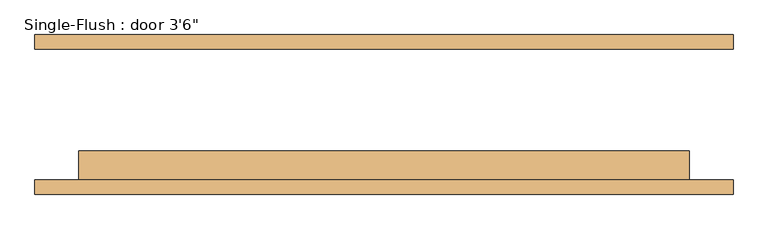
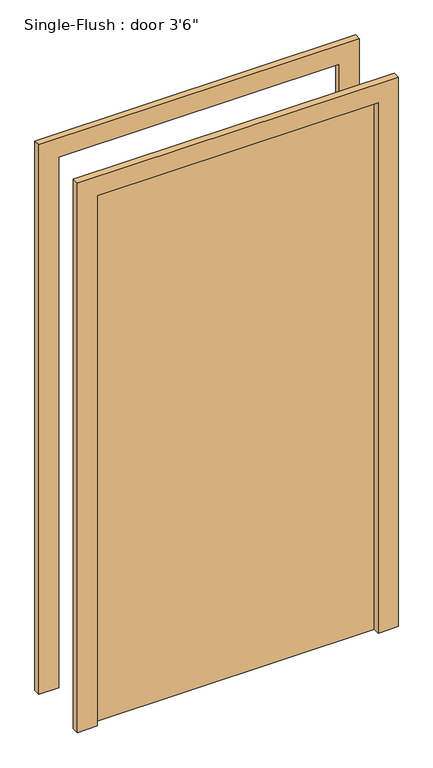
"""IFC4 building model written with IfcOpenShell, lengths in millimetres: door geometry."""

from ifc_helpers import new_model, si_unit, frame, origin, origin_with_axes, place, context, project, spatial, polyline, outline, extrude, source, transform, mapped, element, save


def door_0848dd25(model_context):
    return source(origin(), model_context, "Body", "SweptSolid", [
        extrude(outline(polyline([(2209.8, -609.6), (0.0, -609.6), (0.0, -533.4), (2133.6, -533.4), (2133.6, 533.4), (0.0, 533.4), (0.0, 609.6), (2209.8, 609.6), (2209.8, -609.6)])), frame((0.0, -139.7, 0.0), z_axis=(0.0, 1.0, 0.0), x_axis=(0.0, 0.0, 1.0)), (0.0, 0.0, 1.0), 25.4),
        extrude(outline(polyline([(2209.8, 609.6), (2209.8, -609.6), (0.0, -609.6), (0.0, -533.4), (2133.6, -533.4), (2133.6, 533.4), (0.0, 533.4), (0.0, 609.6), (2209.8, 609.6)])), frame((0.0, 114.3, 0.0), z_axis=(0.0, 1.0, 0.0), x_axis=(0.0, 0.0, 1.0)), (0.0, 0.0, 1.0), 25.4),
        extrude(outline(polyline([(533.4, -63.5), (533.4, -114.3), (-533.4, -114.3), (-533.4, -63.5), (533.4, -63.5)])), origin_with_axes(), (0.0, 0.0, 1.0), 2133.6),
    ])


if __name__ == "__main__":
    model = new_model("IFC4")
    model_context = context("Model", 3, world=origin())
    ifc_project = project(units=[si_unit("LENGTHUNIT", "METRE", prefix="MILLI")], contexts=[model_context])
    site = spatial("IfcSite", under=ifc_project)
    building = spatial("IfcBuilding", under=site)
    placement = place(None, origin())
    door_shape = door_0848dd25(model_context)
    element("IfcDoor", 1, ObjectType="Single-Flush : door 3'6\"", at=placement, inside=building, context=model_context, shape_type="MappedRepresentation", body=[
        mapped(door_shape, transform((0.0, 0.0, 0.0), x_axis=(1.0, 0.0, 0.0), y_axis=(0.0, 1.0, 0.0), z_axis=(0.0, 0.0, 1.0))),
    ])
    save(model, "model.ifc")

# Revit data of these elements
# Type "Single-Flush : door 3'6\""
#   Type Mark = "9"
#   Construction Type Id = "MDOOR"
#   Assembly Code = "C1020"
#   Analytic Construction = "Metal"
#   Thickness = 0' - 2"
#   Heat Transfer Coefficient (U) = 0.651978 BTU/(h·ft²·°F)
#   Height = 7' - 0"
#   Trim Projection Ext = 0' - 1"
#   Trim Projection Int = 0' - 1"
#   Trim Width = 0' - 3"
#   Width = 3' - 6"
#   Define Thermal Properties by = 1
#   Door Material = Door - Panel
#   Frame Material = Door - Frame
#   Visual Light Transmittance = 0
#   Solar Heat Gain Coefficient = 0
#   Function = (empty or 0)
#   Wall Closure = (empty or 0)
# Element 1 (IfcDoor, "Single-Flush : door 3'6\"")
#   Materials on its faces: "Door - Frame", "Door - Panel"
# Materials
#   "Door - Panel": class "Wood", colour RGB 210 159 95, transparency 0, Cost = 0
#   "Door - Frame": colour RGB 118 70 51, transparency 0, Cost = 0
